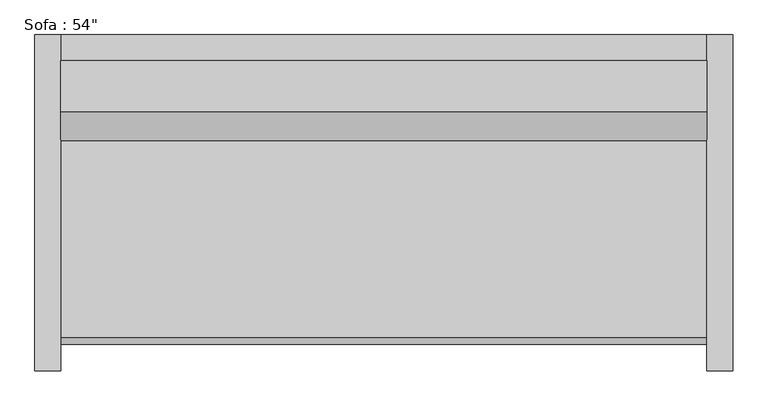
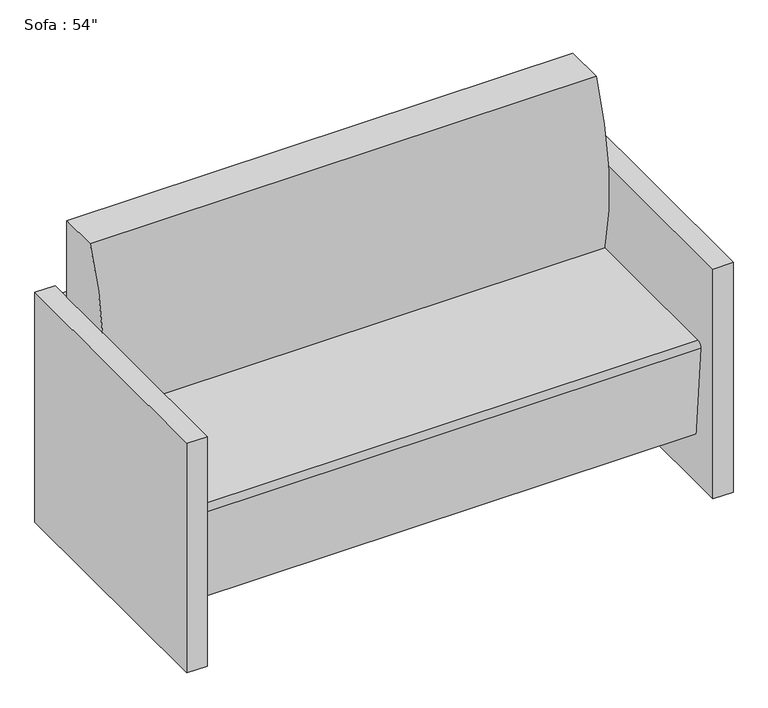
"""IFC4 building model written with IfcOpenShell, lengths in millimetres: furniture geometry."""

from ifc_helpers import new_model, si_unit, point, frame, frame_2d, origin, origin_with_axes, place, context, project, spatial, polyline, circle_curve, trimmed, segment, composite_curve, outline, extrude, source, transform, mapped, element, save


def furniture_22419f35(model_context):
    return source(origin(), model_context, "Body", "SweptSolid", [
        extrude(outline(polyline([(-564.6295082, 425.5540984), (-564.6295082, 476.3540984), (705.3704918, 476.3540984), (705.3704918, 425.5540984), (-564.6295082, 425.5540984)])), frame((0.0, 0.0, 457.2), z_axis=(0.0, 0.0, 1.0), x_axis=(1.0, 0.0, 0.0)), (0.0, 0.0, 1.0), 127.0),
        extrude(outline(polyline([(-564.6295082, 425.5540984), (-564.6295082, 476.3540984), (705.3704918, 476.3540984), (705.3704918, 425.5540984), (-564.6295082, 425.5540984)])), frame((0.0, 0.0, 266.7), z_axis=(0.0, 0.0, 1.0), x_axis=(1.0, 0.0, 0.0)), (0.0, 0.0, 1.0), 127.0),
        extrude(outline(polyline([(-564.6295082, 425.5540984), (-564.6295082, 476.3540984), (705.3704918, 476.3540984), (705.3704918, 425.5540984), (-564.6295082, 425.5540984)])), frame((0.0, 0.0, 76.2), z_axis=(0.0, 0.0, 1.0), x_axis=(1.0, 0.0, 0.0)), (0.0, 0.0, 1.0), 127.0),
        extrude(outline(composite_curve([segment(trimmed(circle_curve(frame_2d((926.517198, 542.5300036)), 660.4), [point((286.1764935, 381.0))], [point((323.9540984, 812.8))], False, "CARTESIAN"), True, "CONTINUOUS"), segment(polyline([(323.9540984, 812.8), (425.5540984, 812.8), (425.5540984, 127.9665467), (-111.108343, 127.9665467), (-132.0379563, 367.1931221)]), True, "CONTINUOUS"), segment(trimmed(circle_curve(frame_2d((-119.3862837, 368.3)), 12.7), [point((-132.0379563, 367.1931221))], [point((-119.3862837, 381.0))], False, "CARTESIAN"), True, "CONTINUOUS"), segment(polyline([(-119.3862837, 381.0), (286.1764935, 381.0)]), True, "CONTINUOUS")], self_intersect=False)), frame((-564.6295082, 0.0, 0.0), z_axis=(1.0, 0.0, 0.0), x_axis=(0.0, 1.0, 0.0)), (0.0, 0.0, 1.0), 1270.0),
        extrude(outline(polyline([(-615.4295082, 476.3540984), (-564.6295082, 476.3540984), (-564.6295082, -184.0459016), (-615.4295082, -184.0459016), (-615.4295082, 476.3540984)])), origin_with_axes(), (0.0, 0.0, 1.0), 609.6),
        extrude(outline(polyline([(756.1704918, 476.3540984), (756.1704918, -184.0459016), (705.3704918, -184.0459016), (705.3704918, 476.3540984), (756.1704918, 476.3540984)])), origin_with_axes(), (0.0, 0.0, 1.0), 609.6),
    ])


if __name__ == "__main__":
    model = new_model("IFC4")
    model_context = context("Model", 3, world=origin())
    ifc_project = project(units=[si_unit("LENGTHUNIT", "METRE", prefix="MILLI")], contexts=[model_context])
    site = spatial("IfcSite", under=ifc_project)
    building = spatial("IfcBuilding", under=site)
    placement = place(None, origin())
    furniture_shape = furniture_22419f35(model_context)
    element("IfcFurniture", 1, ObjectType="Sofa : 54\"", at=placement, inside=building, context=model_context, shape_type="MappedRepresentation", body=[
        mapped(furniture_shape, transform((0.0, 0.0, 0.0), x_axis=(1.0, 0.0, 0.0), y_axis=(0.0, 1.0, 0.0), z_axis=(0.0, 0.0, 1.0))),
    ])
    save(model, "model.ifc")

# Revit data of these elements
# Type "Sofa : 54\""
#   Assembly Code = "E2020200"
#   Width = 4' - 6"
#   Seat Material = none
#   Frame Material = none
#   Default Elevation = 0
# Element 1 (IfcFurniture, "Sofa : 54\"")
#   Materials on its faces: "Cherry"
# Materials
#   "Cherry": class "Wood", colour RGB 226 177 128, transparency 0, Description = "Prunus Serotina", Cost = 0
